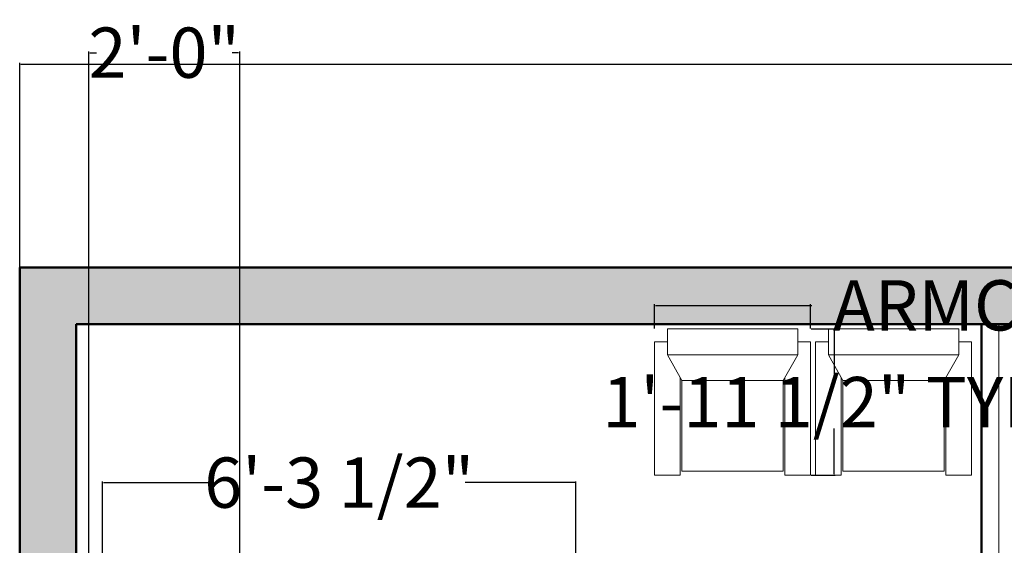
# Model space of a CAD drawing. Units: inches. Extents: x 22042254 to 25404563, y 17568978 to 17626777.
# Tile 41 of 45: x 22179784 to 22179940, y 17626694 to 17626777. Entities that reach past the tile are written whole.
import ezdxf

# ---------------------------------------------------------------- set-up
doc = ezdxf.new("R2010")
doc.units = ezdxf.units.IN
doc.header["$MEASUREMENT"] = 0
for name, color, linetype, lineweight in [('A-ANNO-DIMS', 2, 'Continuous', 18), ('A-FLOR-OPEN', 252, 'Continuous', 18), ('A-WALL-PATT', 244, 'Continuous', 13), ('furniture', 8, 'Continuous', 18), ('walls', 252, 'Continuous', 50)]:
    doc.layers.add(name, color=color, linetype=linetype, lineweight=lineweight)
doc.styles.get("Standard").update_dxf_attribs({"font": 'arial.ttf'})
doc.dimstyles.get("Standard").update_dxf_attribs({"dimtxt": 8, "dimasz": 0.18, "dimexe": 0.18, "dimexo": 0.0625, "dimgap": 0.09, "dimtad": 0, "dimtih": 1, "dimtoh": 1, "dimzin": 0, "dimdsep": 46, "dimlunit": 3, "dimtxsty": 'Standard', "dimcen": 0.09, "dimadec": 0, "dimazin": 0, "dimtfac": 1, "dimtofl": 0, "dimtmove": 0, "dimatfit": 3, "dimfxl": 1, "dimtolj": 1, "dimtzin": 0, "dimarcsym": 0})

# ---------------------------------------------------------------- blocks, each defined once
blk = doc.blocks.new('*D1')
at = {"layer": 'A-ANNO-DIMS', "color": 0, "lineweight": -2, "transparency": 16777216}
for p, q in [((22179783.73, 17626737.84), (22179783.73, 17626770.35)), ((22179783.91, 17626770.17), (22179956.86, 17626770.17)), ((22180143.55, 17626770.17), (22179970.61, 17626770.17)), ((22180143.73, 17626737.84), (22180143.73, 17626770.35))]:
    blk.add_line(p, q, dxfattribs=at)
at = {"layer": 'A-ANNO-DIMS', "color": 0, "transparency": 16777216}
for points in [[(22179783.91, 17626770.2), (22179783.91, 17626770.14), (22179783.73, 17626770.17)], [(22180143.55, 17626770.2), (22180143.55, 17626770.14), (22180143.73, 17626770.17)]]:
    blk.add_solid(points, dxfattribs=at)
at = {"layer": 'Defpoints', "color": 0, "transparency": 16777216}
for p in [(22180143.73, 17626770.17), (22179783.73, 17626737.78), (22180143.73, 17626737.78)]:
    blk.add_point(p, dxfattribs=at)
at = {"layer": 'A-ANNO-DIMS', "color": 0, "transparency": 16777216, "insert": (22179963.73, 17626770.17), "char_height": 8, "attachment_point": 5}
blk.add_mtext("\\A1;30'", dxfattribs=at)
blk = doc.blocks.new('FABRIC SOFA 1S')
at = {"layer": 'furniture'}
for p, q in [((3, 18.12), (34, 18.12)), ((3, 15.12), (3, 18.12)), ((34, 12.12), (34, 18.12)), ((0, -15.12), (0, 15.12)), ((6, 15.12), (0, 15.12)), ((6, -15.12), (6, 15.12)), ((12, 11.75), (6, 15.12)), ((11.33, 12.12), (34, 12.12)), ((6, -15.12), (12, -11.75)), ((11.33, -12.12), (34, -12.12)), ((34, -12.12), (34, -18.12)), ((6, -15.12), (0, -15.12)), ((3, -18.12), (3, -15.12)), ((3, -18.12), (34, -18.12))]:
    blk.add_line(p, q, dxfattribs=at)
blk.add_lwpolyline([(12, -11.75), (12, 11.75), (33, 11.75), (33, -11.75)], close=True, dxfattribs=at)
blk = doc.blocks.new('*D31')
at = {"layer": 'A-ANNO-DIMS', "color": 0, "lineweight": -2, "transparency": 16777216}
for p, q in [((22179796.91, 17626691.28), (22179796.91, 17626703.76)), ((22179797.09, 17626703.58), (22179814.48, 17626703.58)), ((22179872.01, 17626703.58), (22179854.61, 17626703.58)), ((22179872.19, 17626691.28), (22179872.19, 17626703.76))]:
    blk.add_line(p, q, dxfattribs=at)
at = {"layer": 'A-ANNO-DIMS', "color": 0, "transparency": 16777216}
for points in [[(22179797.09, 17626703.61), (22179797.09, 17626703.55), (22179796.91, 17626703.58)], [(22179872.01, 17626703.61), (22179872.01, 17626703.55), (22179872.19, 17626703.58)]]:
    blk.add_solid(points, dxfattribs=at)
at = {"layer": 'Defpoints', "color": 0, "transparency": 16777216}
for p in [(22179872.19, 17626703.58), (22179796.91, 17626691.22), (22179872.19, 17626691.22)]:
    blk.add_point(p, dxfattribs=at)
at = {"layer": 'A-ANNO-DIMS', "color": 0, "transparency": 16777216, "insert": (22179834.55, 17626703.58), "char_height": 8, "attachment_point": 5}
blk.add_mtext('\\A1;6\'-3 1/2"', dxfattribs=at)
blk = doc.blocks.new('*D36')
at = {"layer": 'A-ANNO-DIMS', "color": 0, "lineweight": -2, "transparency": 16777216}
for p, q in [((22179884.69, 17626728.11), (22179884.69, 17626731.96)), ((22179884.87, 17626731.78), (22179909.36, 17626731.78)), ((22179909.54, 17626728.11), (22179909.54, 17626731.96)), ((22179909.54, 17626731.78), (22179909.72, 17626731.78))]:
    blk.add_line(p, q, dxfattribs=at)
at = {"layer": 'A-ANNO-DIMS', "color": 0, "transparency": 16777216}
for points in [[(22179884.87, 17626731.81), (22179884.87, 17626731.75), (22179884.69, 17626731.78)], [(22179909.36, 17626731.81), (22179909.36, 17626731.75), (22179909.54, 17626731.78)]]:
    blk.add_solid(points, dxfattribs=at)
at = {"layer": 'Defpoints', "color": 0, "transparency": 16777216}
for p in [(22179909.54, 17626731.78), (22179884.69, 17626728.05), (22179909.54, 17626728.05)]:
    blk.add_point(p, dxfattribs=at)
at = {"layer": 'A-ANNO-DIMS', "color": 0, "transparency": 16777216, "insert": (22179965.78, 17626731.78), "char_height": 8, "attachment_point": 5}
blk.add_mtext('\\A1;ARMCHAIR 2\'-1" TYP.', dxfattribs=at)
blk = doc.blocks.new('*D37')
at = {"layer": 'A-ANNO-DIMS', "color": 0, "lineweight": -2, "transparency": 16777216}
for p, q in [((22179909.6, 17626728.05), (22179913.44, 17626728.05)), ((22179913.26, 17626727.87), (22179913.26, 17626720.62)), ((22179913.26, 17626704.92), (22179913.26, 17626712.17)), ((22179909.6, 17626704.74), (22179913.44, 17626704.74))]:
    blk.add_line(p, q, dxfattribs=at)
at = {"layer": 'A-ANNO-DIMS', "color": 0, "transparency": 16777216}
for points in [[(22179913.23, 17626727.87), (22179913.29, 17626727.87), (22179913.26, 17626728.05)], [(22179913.23, 17626704.92), (22179913.29, 17626704.92), (22179913.26, 17626704.74)]]:
    blk.add_solid(points, dxfattribs=at)
at = {"layer": 'Defpoints', "color": 0, "transparency": 16777216}
for p in [(22179909.54, 17626728.05), (22179909.54, 17626704.74), (22179913.26, 17626704.74)]:
    blk.add_point(p, dxfattribs=at)
at = {"layer": 'A-ANNO-DIMS', "color": 0, "transparency": 16777216, "insert": (22179913.26, 17626716.39), "char_height": 8, "attachment_point": 5}
blk.add_mtext('\\A1;1\'-11 1/2" TYP.', dxfattribs=at)
blk = doc.blocks.new('*D60')
at = {"layer": 'A-ANNO-DIMS', "color": 0, "lineweight": -2, "transparency": 16777216}
for p, q in [((22179794.73, 17626555.5), (22179794.73, 17626772.16)), ((22179794.91, 17626771.98), (22179795.94, 17626771.98)), ((22179818.55, 17626771.98), (22179817.52, 17626771.98)), ((22179818.73, 17626560), (22179818.73, 17626772.16))]:
    blk.add_line(p, q, dxfattribs=at)
at = {"layer": 'A-ANNO-DIMS', "color": 0, "transparency": 16777216}
for points in [[(22179794.91, 17626772.01), (22179794.91, 17626771.95), (22179794.73, 17626771.98)], [(22179818.55, 17626772.01), (22179818.55, 17626771.95), (22179818.73, 17626771.98)]]:
    blk.add_solid(points, dxfattribs=at)
at = {"layer": 'Defpoints', "color": 0, "transparency": 16777216}
for p in [(22179818.73, 17626771.98), (22179818.73, 17626559.94), (22179794.73, 17626555.44)]:
    blk.add_point(p, dxfattribs=at)
at = {"layer": 'A-ANNO-DIMS', "color": 0, "transparency": 16777216, "insert": (22179806.73, 17626771.98), "char_height": 8, "attachment_point": 5}
blk.add_mtext('\\A1;2\'-0"', dxfattribs=at)

msp = doc.modelspace()

# ---------------------------------------------------------------- hatches: boundary and pattern name
at = {"layer": 'A-WALL-PATT'}
h = msp.add_hatch(color=256, dxfattribs=at)
h.dxf.hatch_style = 1
h.paths.add_polyline_path([(22179792.734, 17626580.28), (22179888.734, 17626580.28), (22179888.734, 17626559.623), (22179893.234, 17626559.623), (22179893.234, 17626580.28), (22179900.438, 17626580.28), (22179900.438, 17626584.78), (22179792.734, 17626584.78), (22179792.734, 17626728.78), (22180134.734, 17626728.78), (22180134.734, 17626584.78), (22180035.602, 17626584.78), (22180004.432, 17626584.78), (22180001.734, 17626584.78), (22180001.734, 17626580.28), (22180134.734, 17626580.28), (22180134.734, 17626404.28), (22180064.487, 17626404.28), (22180064.487, 17626399.78), (22180134.734, 17626399.78), (22180134.734, 17626197.78), (22180143.734, 17626197.78), (22180143.734, 17626737.78), (22179783.734, 17626737.78), (22179783.734, 17626197.78), (22179792.734, 17626197.78), (22179792.734, 17626394.78), (22179936.734, 17626394.78), (22179936.734, 17626383.208), (22179941.234, 17626383.208), (22179941.234, 17626532.28), (22179927.066, 17626532.28), (22179927.066, 17626527.78), (22179928.072, 17626527.78), (22179936.734, 17626527.78), (22179936.734, 17626403.78), (22179792.734, 17626403.78), (22179792.734, 17626527.78), (22179905.094, 17626527.78), (22179905.094, 17626532.28), (22179792.734, 17626532.28)])

# ---------------------------------------------------------------- linework, layer by layer
at = {"layer": 'A-FLOR-OPEN'}
msp.add_line((22179939.449, 17626680.78), (22179939.449, 17626728.78), dxfattribs=at)
at = {"layer": 'walls'}
for p, q in [((22179783.734, 17626737.78), (22180143.734, 17626737.78)), ((22179783.734, 17626197.78), (22179783.734, 17626737.78)), ((22179783.734, 17626737.78), (22179783.734, 17626737.78)), ((22179792.734, 17626728.78), (22180134.734, 17626728.78)), ((22179792.734, 17626584.78), (22179792.734, 17626728.78)), ((22179936.734, 17626580.28), (22179936.734, 17626728.78))]:
    msp.add_line(p, q, dxfattribs=at)

# ---------------------------------------------------------------- block references
at = {"layer": 'furniture', "xscale": 0.685544738852578, "yscale": 0.685544738852578, "zscale": 0.685544738852578, "rotation": 270}
for p in [(22179897.112, 17626728.048), (22179922.72, 17626728.048)]:
    msp.add_blockref('FABRIC SOFA 1S', p, dxfattribs=at)

# ---------------------------------------------------------------- dimensions: what is measured, and where the dimension line sits
at = {"layer": 'A-ANNO-DIMS'}
for base, p1, p2, override, picture, middle in [((22179818.734, 17626771.98), (22179794.734, 17626555.436), (22179818.734, 17626559.936), {"dimdec": 1, "dimlfac": 1, "dimrnd": 0, "dimzin": 1, "dimdsep": 46, "dimlunit": 4, "dimfrac": 2}, '*D60', (22179806.734, 17626771.98)), ((22180143.734, 17626770.174), (22179783.734, 17626737.78), (22180143.734, 17626737.78), {"dimclrd": 0, "dimclre": 0, "dimclrt": 0}, '*D1', (22179963.734, 17626770.174)), ((22179872.186, 17626703.578), (22179796.907, 17626691.22), (22179872.186, 17626691.22), {"dimdec": 1, "dimlfac": 1, "dimrnd": 0, "dimzin": 1, "dimdsep": 46, "dimlunit": 4, "dimfrac": 2}, '*D31', (22179834.546, 17626703.578))]:
    dim = msp.add_linear_dim(base=base, p1=p1, p2=p2, dimstyle='Standard', override=override, dxfattribs=at)
    dim.commit()
    dim.dimension.update_dxf_attribs({"geometry": picture, "text_midpoint": middle})
dim = msp.add_linear_dim(base=(22179909.537, 17626731.776), p1=(22179884.686, 17626728.048), p2=(22179909.537, 17626728.048), text='ARMCHAIR <> TYP.', dimstyle='Standard', override={"dimdec": 1, "dimlfac": 1, "dimrnd": 0, "dimzin": 1, "dimdsep": 46, "dimlunit": 4, "dimfrac": 2}, dxfattribs=at)
dim.commit()
dim.dimension.update_dxf_attribs({"geometry": '*D36', "text_midpoint": (22179965.777, 17626731.776)})
dim = msp.add_linear_dim(base=(22179913.265, 17626704.74), p1=(22179909.537, 17626728.048), p2=(22179909.537, 17626704.74), angle=270, text='<> TYP.', dimstyle='Standard', override={"dimdec": 1, "dimlfac": 1, "dimrnd": 0, "dimzin": 1, "dimdsep": 46, "dimlunit": 4, "dimfrac": 2}, dxfattribs=at)
dim.commit()
dim.dimension.update_dxf_attribs({"geometry": '*D37', "text_midpoint": (22179913.265, 17626716.394)})

doc.saveas('drawing.dxf')
